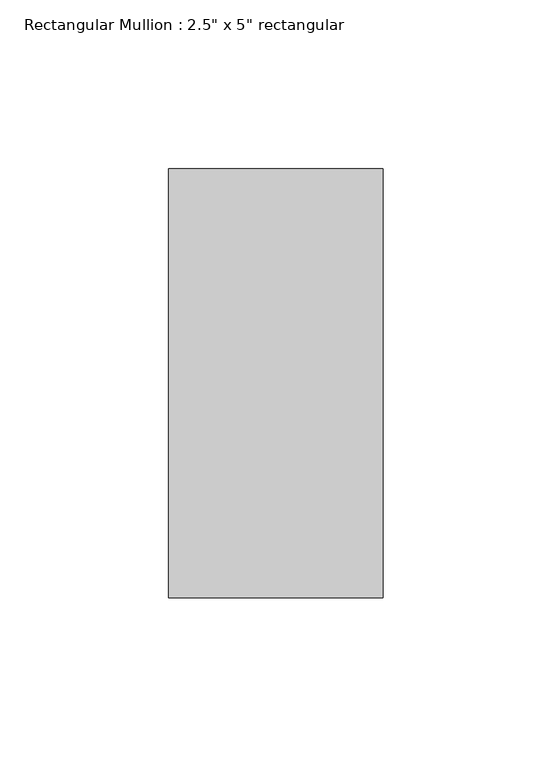
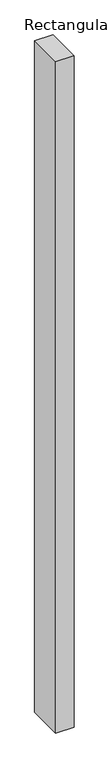
"""IFC4 building model written with IfcOpenShell, lengths in millimetres: member geometry."""

from ifc_helpers import new_model, si_unit, frame, origin, place, context, project, spatial, polyline, outline, extrude, source, transform, mapped, element, save


def member_0537779b(model_context):
    return source(origin(), model_context, "Body", "SweptSolid", [
        extrude(outline(polyline([(0.0, 63.5), (0.0, -63.5), (-63.5, -63.5), (-63.5, 63.5), (0.0, 63.5)])), frame((0.0, 0.0, -2468.3449309), z_axis=(0.0, 0.0, 1.0), x_axis=(1.0, 0.0, 0.0)), (0.0, 0.0, 1.0), 2468.3449309),
    ])


if __name__ == "__main__":
    model = new_model("IFC4")
    model_context = context("Model", 3, world=origin())
    ifc_project = project(units=[si_unit("LENGTHUNIT", "METRE", prefix="MILLI")], contexts=[model_context])
    site = spatial("IfcSite", under=ifc_project)
    building = spatial("IfcBuilding", under=site)
    placement = place(None, origin())
    member_shape = member_0537779b(model_context)
    element("IfcMember", 1, ObjectType="Rectangular Mullion : 2.5\" x 5\" rectangular", at=placement, inside=building, context=model_context, shape_type="MappedRepresentation", body=[
        mapped(member_shape, transform((0.0, 0.0, 0.0), x_axis=(1.0, 0.0, 0.0), y_axis=(0.0, 1.0, 0.0), z_axis=(0.0, 0.0, 1.0))),
    ])
    save(model, "model.ifc")

# Revit data of these elements
# Type "Rectangular Mullion : 2.5\" x 5\" rectangular"
#   built-in parameter 1007304 = 0.416667 (stored number, unit not read)
#   built-in parameter 1007301 = 0.104167 (stored number, unit not read)
#   built-in parameter 1007300 = 0.104167 (stored number, unit not read)
# Element 1 (IfcMember, "Rectangular Mullion : 2.5\" x 5\" rectangular")
#   Materials on its faces: "Aluminum"
# Materials
#   "Aluminum": class "Metal", colour RGB 247 247 247, transparency 0, Description = "Aluminum 6061", Cost = 0
